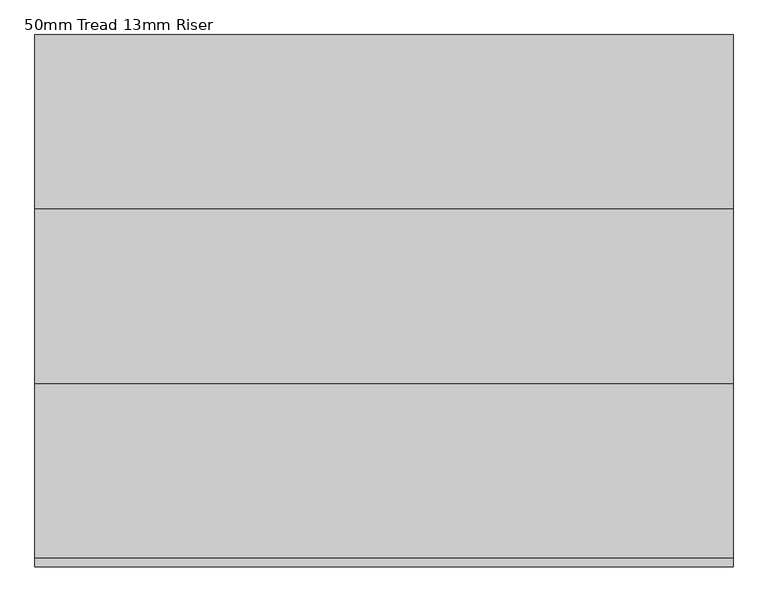
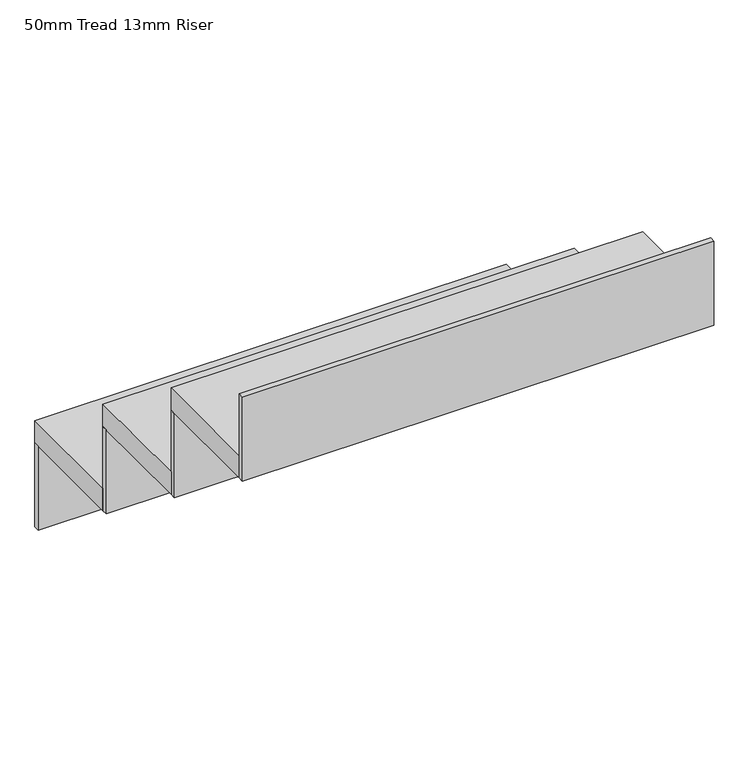
"""IFC4 building model written with IfcOpenShell, lengths in millimetres: stair flight geometry, 50mm Tread 13mm Riser."""

from ifc_helpers import new_model, si_unit, frame, origin, place, context, project, spatial, polyline, outline, extrude, source, transform, mapped, element, save


def stair_flight_50mm_tread_13mm_riser_ddd89fd2(model_context):
    return source(origin(), model_context, "Body", "SweptSolid", [
        extrude(outline(polyline([(-10477.6052721, -2511.0618509), (-10477.6052721, -2498.5618509), (-9477.5794909, -2498.5618509), (-9477.5794909, -2511.0618509), (-10477.6052721, -2511.0618509)])), frame((0.0, 0.0, 10869.0117647), z_axis=(0.0, 0.0, 1.0), x_axis=(1.0, 0.0, 0.0)), (0.0, 0.0, 1.0), 188.2588235),
        extrude(outline(polyline([(-9477.5794909, -2748.5618509), (-10477.6052721, -2748.5618509), (-10477.6052721, -2498.5618509), (-9477.5794909, -2498.5618509), (-9477.5794909, -2748.5618509)])), frame((0.0, 0.0, 11057.2705882), z_axis=(0.0, 0.0, 1.0), x_axis=(1.0, 0.0, 0.0)), (0.0, 0.0, 1.0), 50.0),
        extrude(outline(polyline([(-10477.6052721, -2761.0618509), (-10477.6052721, -2748.5618509), (-9477.5794909, -2748.5618509), (-9477.5794909, -2761.0618509), (-10477.6052721, -2761.0618509)])), frame((0.0, 0.0, 11057.2705882), z_axis=(0.0, 0.0, 1.0), x_axis=(1.0, 0.0, 0.0)), (0.0, 0.0, 1.0), 188.2588235),
        extrude(outline(polyline([(-9477.5794909, -2998.5618509), (-10477.6052721, -2998.5618509), (-10477.6052721, -2748.5618509), (-9477.5794909, -2748.5618509), (-9477.5794909, -2998.5618509)])), frame((0.0, 0.0, 11245.5294118), z_axis=(0.0, 0.0, 1.0), x_axis=(1.0, 0.0, 0.0)), (0.0, 0.0, 1.0), 50.0),
        extrude(outline(polyline([(-10477.6052721, -3011.0618509), (-10477.6052721, -2998.5618509), (-9477.5794909, -2998.5618509), (-9477.5794909, -3011.0618509), (-10477.6052721, -3011.0618509)])), frame((0.0, 0.0, 11245.5294118), z_axis=(0.0, 0.0, 1.0), x_axis=(1.0, 0.0, 0.0)), (0.0, 0.0, 1.0), 188.2588235),
        extrude(outline(polyline([(-10477.6052721, -3261.0618509), (-10477.6052721, -3248.5618509), (-9477.5794909, -3248.5618509), (-9477.5794909, -3261.0618509), (-10477.6052721, -3261.0618509)])), frame((0.0, 0.0, 11433.7882353), z_axis=(0.0, 0.0, 1.0), x_axis=(1.0, 0.0, 0.0)), (0.0, 0.0, 1.0), 188.2588235),
        extrude(outline(polyline([(-9477.5794909, -3248.5618509), (-10477.6052721, -3248.5618509), (-10477.6052721, -2998.5618509), (-9477.5794909, -2998.5618509), (-9477.5794909, -3248.5618509)])), frame((0.0, 0.0, 11433.7882353), z_axis=(0.0, 0.0, 1.0), x_axis=(1.0, 0.0, 0.0)), (0.0, 0.0, 1.0), 50.0),
    ])


if __name__ == "__main__":
    model = new_model("IFC4")
    model_context = context("Model", 3, world=origin())
    ifc_project = project(units=[si_unit("LENGTHUNIT", "METRE", prefix="MILLI")], contexts=[model_context])
    site = spatial("IfcSite", under=ifc_project)
    building = spatial("IfcBuilding", under=site)
    placement = place(None, origin())
    stair_flight_50mm_tread_13mm_riser_shape = stair_flight_50mm_tread_13mm_riser_ddd89fd2(model_context)
    element("IfcStairFlight", 1, ObjectType="50mm Tread 13mm Riser", at=placement, inside=building, context=model_context, shape_type="MappedRepresentation", body=[
        mapped(stair_flight_50mm_tread_13mm_riser_shape, transform((0.0, 0.0, 0.0), x_axis=(1.0, 0.0, 0.0), y_axis=(0.0, 1.0, 0.0), z_axis=(0.0, 0.0, 1.0))),
    ])
    save(model, "model.ifc")
